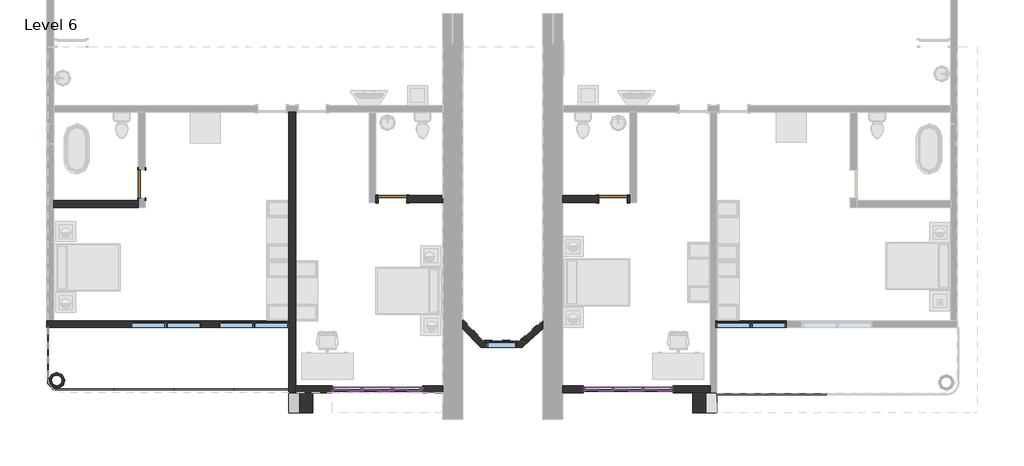
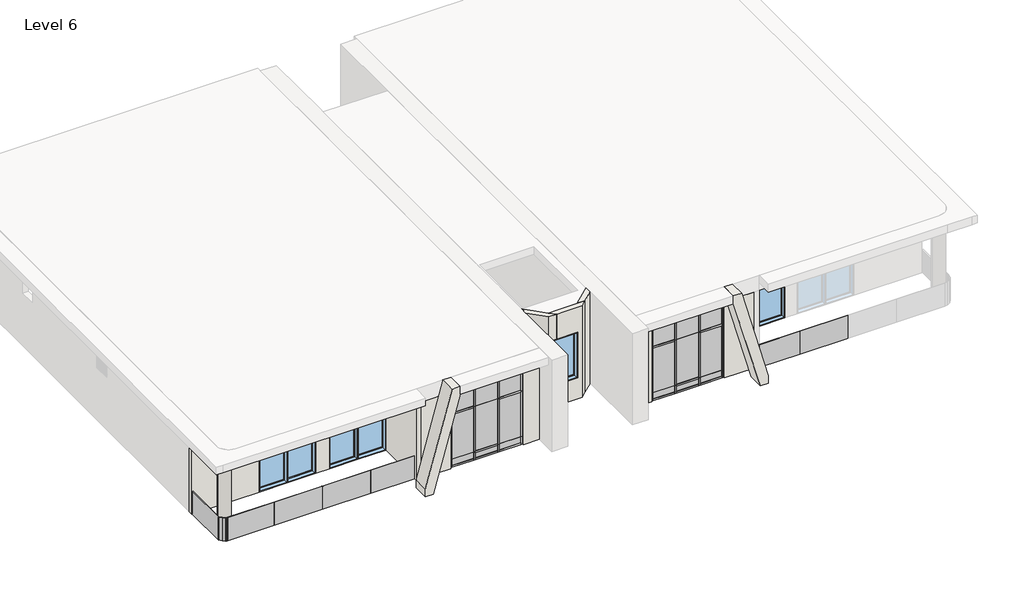
# One storey, part 1 of 3: 42 members, 29 plates, 16 walls, 7 windows, 3 doors.
"""IFC4 building model written with IfcOpenShell, lengths in millimetres."""

from ifc_helpers import new_model, si_unit, point, frame, frame_2d, origin, place, context, project, spatial, polyline, circle_curve, trimmed, segment, composite_curve, outline, extrude, faceted_brep, transform, mapped, element, save
from components import door_2703ae13, door_10fd3a06, member_c17f1be2, member_ad567e07, member_d2e7e466, member_7db1855a, member_75d1e245, member_d60e8053, member_3c3dc66a, member_2fae0574, member_410c6227, member_73c23c35, system_panel_glazed_38d54ecf, system_panel_glazed_fbb6c980, system_panel_glazed_4137532c, system_panel_glazed_6230de04, system_panel_glazed_a79f7f85, system_panel_glazed_9a5ea490, system_panel_glazed_95be5de7, system_panel_glazed_ffe51582, system_panel_glazed_8f95e3f6, system_panel_glazed_836907cd, system_panel_glazed_688a65a2, system_panel_glazed_c1a1c740, system_panel_glazed_22bcd51f, system_panel_glazed_4be86f7f, window_9a779fa2, window_1a213a25

model = new_model("IFC4")

# Units and contexts
model_context = context("Model", 3, world=origin())
ifc_project = project(units=[si_unit("LENGTHUNIT", "METRE", prefix="MILLI")], contexts=[model_context])

# Site, building, storey
site = spatial("IfcSite", under=ifc_project)
building = spatial("IfcBuilding", under=site)
storey = spatial("IfcBuildingStorey", under=building, Name="Level 6", Elevation=18288.0)

# Doors
placement = place(None, origin())
door_shape = door_2703ae13(model_context)
element("IfcDoor", 1, ObjectType="Door-Single-Panel.0001 : 34\" x 80\"", at=placement, inside=storey, context=model_context, shape_type="MappedRepresentation", body=[
    mapped(door_shape, transform((-15765.9987704, -441.9241442, 18288.0), x_axis=(0.0, -1.0, 0.0), y_axis=(1.0, 0.0, 0.0), z_axis=(0.0, 0.0, 1.0))),
])
element("IfcDoor", 2, ObjectType="Door-Single-Panel.0001 : 34\" x 80\"", at=placement, inside=storey, context=model_context, shape_type="MappedRepresentation", body=[
    mapped(door_shape, transform((-8145.9987704, -899.1241442, 18288.0), x_axis=(-1.0, 0.0, 0.0), y_axis=(0.0, -1.0, 0.0), z_axis=(0.0, 0.0, 1.0))),
])
door_2_shape = door_10fd3a06(model_context)
element("IfcDoor", 3, ObjectType="Door-Single-Panel.0001 : 34\" x 80\"", at=placement, inside=storey, context=model_context, shape_type="MappedRepresentation", body=[
    mapped(door_2_shape, transform((-1440.3987704, -899.1241442, 18288.0), x_axis=(1.0, 0.0, 0.0), y_axis=(0.0, 1.0, 0.0), z_axis=(0.0, 0.0, 1.0))),
])

# Members
member_shape = member_c17f1be2(model_context)
element("IfcMember", 4, ObjectType="Rectangular Mullion : 2.5\" x 5\" rectangular", at=placement, inside=storey, context=model_context, shape_type="MappedRepresentation", body=[
    mapped(member_shape, transform((-9911.2987704, -6690.3241442, 21336.0), x_axis=(0.0, 0.0, 1.0), y_axis=(0.0, 1.0, 0.0), z_axis=(-1.0, 0.0, 0.0))),
])
element("IfcMember", 5, ObjectType="Rectangular Mullion : 2.5\" x 5\" rectangular", at=placement, inside=storey, context=model_context, shape_type="MappedRepresentation", body=[
    mapped(member_shape, transform((-8114.2487704, -6690.3241442, 21336.0), x_axis=(0.0, 0.0, 1.0), y_axis=(0.0, 1.0, 0.0), z_axis=(-1.0, 0.0, 0.0))),
])
element("IfcMember", 6, ObjectType="Rectangular Mullion : 2.5\" x 5\" rectangular", at=placement, inside=storey, context=model_context, shape_type="MappedRepresentation", body=[
    mapped(member_shape, transform((-2291.2987704, -6690.3241442, 21336.0), x_axis=(0.0, 0.0, 1.0), y_axis=(0.0, 1.0, 0.0), z_axis=(-1.0, 0.0, 0.0))),
])
element("IfcMember", 7, ObjectType="Rectangular Mullion : 2.5\" x 5\" rectangular", at=placement, inside=storey, context=model_context, shape_type="MappedRepresentation", body=[
    mapped(member_shape, transform((-494.2487704, -6690.3241442, 21336.0), x_axis=(0.0, 0.0, 1.0), y_axis=(0.0, 1.0, 0.0), z_axis=(-1.0, 0.0, 0.0))),
])
element("IfcMember", 8, ObjectType="Rectangular Mullion : 2.5\" x 5\" rectangular", at=placement, inside=storey, context=model_context, shape_type="MappedRepresentation", body=[
    mapped(member_shape, transform((-7295.0987704, -6690.3241442, 18288.0), x_axis=(0.0, 0.0, -1.0), y_axis=(0.0, 1.0, 0.0), z_axis=(1.0, 0.0, 0.0))),
])
element("IfcMember", 9, ObjectType="Rectangular Mullion : 2.5\" x 5\" rectangular", at=placement, inside=storey, context=model_context, shape_type="MappedRepresentation", body=[
    mapped(member_shape, transform((-9092.1487704, -6690.3241442, 18288.0), x_axis=(0.0, 0.0, -1.0), y_axis=(0.0, 1.0, 0.0), z_axis=(1.0, 0.0, 0.0))),
])
element("IfcMember", 10, ObjectType="Rectangular Mullion : 2.5\" x 5\" rectangular", at=placement, inside=storey, context=model_context, shape_type="MappedRepresentation", body=[
    mapped(member_shape, transform((324.9012296, -6690.3241442, 18288.0), x_axis=(0.0, 0.0, -1.0), y_axis=(0.0, 1.0, 0.0), z_axis=(1.0, 0.0, 0.0))),
])
element("IfcMember", 11, ObjectType="Rectangular Mullion : 2.5\" x 5\" rectangular", at=placement, inside=storey, context=model_context, shape_type="MappedRepresentation", body=[
    mapped(member_shape, transform((-1472.1487704, -6690.3241442, 18288.0), x_axis=(0.0, 0.0, -1.0), y_axis=(0.0, 1.0, 0.0), z_axis=(1.0, 0.0, 0.0))),
])
member_2_shape = member_ad567e07(model_context)
element("IfcMember", 12, ObjectType="Rectangular Mullion : 2.5\" x 5\" rectangular", at=placement, inside=storey, context=model_context, shape_type="MappedRepresentation", body=[
    mapped(member_2_shape, transform((-8114.2487704, -6690.3241442, 20421.6), x_axis=(0.0, 0.0, 1.0), y_axis=(0.0, 1.0, 0.0), z_axis=(-1.0, 0.0, 0.0))),
])
element("IfcMember", 13, ObjectType="Rectangular Mullion : 2.5\" x 5\" rectangular", at=placement, inside=storey, context=model_context, shape_type="MappedRepresentation", body=[
    mapped(member_2_shape, transform((-9911.2987704, -6690.3241442, 20421.6), x_axis=(0.0, 0.0, 1.0), y_axis=(0.0, 1.0, 0.0), z_axis=(-1.0, 0.0, 0.0))),
])
element("IfcMember", 14, ObjectType="Rectangular Mullion : 2.5\" x 5\" rectangular", at=placement, inside=storey, context=model_context, shape_type="MappedRepresentation", body=[
    mapped(member_2_shape, transform((-494.2487704, -6690.3241442, 20421.6), x_axis=(0.0, 0.0, 1.0), y_axis=(0.0, 1.0, 0.0), z_axis=(-1.0, 0.0, 0.0))),
])
element("IfcMember", 15, ObjectType="Rectangular Mullion : 2.5\" x 5\" rectangular", at=placement, inside=storey, context=model_context, shape_type="MappedRepresentation", body=[
    mapped(member_2_shape, transform((-2291.2987704, -6690.3241442, 20421.6), x_axis=(0.0, 0.0, 1.0), y_axis=(0.0, 1.0, 0.0), z_axis=(-1.0, 0.0, 0.0))),
])
member_3_shape = member_d2e7e466(model_context)
element("IfcMember", 16, ObjectType="Rectangular Mullion : 2.5\" x 5\" rectangular", at=placement, inside=storey, context=model_context, shape_type="MappedRepresentation", body=[
    mapped(member_3_shape, transform((-8177.7487704, -6690.3241442, 18288.0), x_axis=(0.0, 0.0, -1.0), y_axis=(0.0, 1.0, 0.0), z_axis=(1.0, 0.0, 0.0))),
])
element("IfcMember", 17, ObjectType="Rectangular Mullion : 2.5\" x 5\" rectangular", at=placement, inside=storey, context=model_context, shape_type="MappedRepresentation", body=[
    mapped(member_3_shape, transform((-557.7487704, -6690.3241442, 18288.0), x_axis=(0.0, 0.0, -1.0), y_axis=(0.0, 1.0, 0.0), z_axis=(1.0, 0.0, 0.0))),
])
member_4_shape = member_7db1855a(model_context)
element("IfcMember", 18, ObjectType="Rectangular Mullion : 2.5\" x 5\" rectangular", at=placement, inside=storey, context=model_context, shape_type="MappedRepresentation", body=[
    mapped(member_4_shape, transform((-9028.6487704, -6690.3241442, 18592.8), x_axis=(0.0, 0.0, 1.0), y_axis=(0.0, 1.0, 0.0), z_axis=(-1.0, 0.0, 0.0))),
])
element("IfcMember", 19, ObjectType="Rectangular Mullion : 2.5\" x 5\" rectangular", at=placement, inside=storey, context=model_context, shape_type="MappedRepresentation", body=[
    mapped(member_4_shape, transform((-1408.6487704, -6690.3241442, 18592.8), x_axis=(0.0, 0.0, 1.0), y_axis=(0.0, 1.0, 0.0), z_axis=(-1.0, 0.0, 0.0))),
])
element("IfcMember", 20, ObjectType="Rectangular Mullion : 2.5\" x 5\" rectangular", at=placement, inside=storey, context=model_context, shape_type="MappedRepresentation", body=[
    mapped(member_3_shape, transform((-9028.6487704, -6690.3241442, 21336.0), x_axis=(0.0, 0.0, 1.0), y_axis=(0.0, 1.0, 0.0), z_axis=(-1.0, 0.0, 0.0))),
])
element("IfcMember", 21, ObjectType="Rectangular Mullion : 2.5\" x 5\" rectangular", at=placement, inside=storey, context=model_context, shape_type="MappedRepresentation", body=[
    mapped(member_3_shape, transform((-1408.6487704, -6690.3241442, 21336.0), x_axis=(0.0, 0.0, 1.0), y_axis=(0.0, 1.0, 0.0), z_axis=(-1.0, 0.0, 0.0))),
])
member_5_shape = member_75d1e245(model_context)
element("IfcMember", 22, ObjectType="Rectangular Mullion : 2.5\" x 5\" rectangular", at=placement, inside=storey, context=model_context, shape_type="MappedRepresentation", body=[
    mapped(member_5_shape, transform((-8145.9987704, -6690.3241442, 18288.0), x_axis=(-1.0, 0.0, 0.0), y_axis=(0.0, 1.0, 0.0), z_axis=(0.0, 0.0, -1.0))),
])
element("IfcMember", 23, ObjectType="Rectangular Mullion : 2.5\" x 5\" rectangular", at=placement, inside=storey, context=model_context, shape_type="MappedRepresentation", body=[
    mapped(member_5_shape, transform((-9060.3987704, -6690.3241442, 18288.0), x_axis=(-1.0, 0.0, 0.0), y_axis=(0.0, 1.0, 0.0), z_axis=(0.0, 0.0, -1.0))),
])
element("IfcMember", 24, ObjectType="Rectangular Mullion : 2.5\" x 5\" rectangular", at=placement, inside=storey, context=model_context, shape_type="MappedRepresentation", body=[
    mapped(member_5_shape, transform((-525.9987704, -6690.3241442, 18288.0), x_axis=(-1.0, 0.0, 0.0), y_axis=(0.0, 1.0, 0.0), z_axis=(0.0, 0.0, -1.0))),
])
element("IfcMember", 25, ObjectType="Rectangular Mullion : 2.5\" x 5\" rectangular", at=placement, inside=storey, context=model_context, shape_type="MappedRepresentation", body=[
    mapped(member_5_shape, transform((-1440.3987704, -6690.3241442, 18288.0), x_axis=(-1.0, 0.0, 0.0), y_axis=(0.0, 1.0, 0.0), z_axis=(0.0, 0.0, -1.0))),
])
member_6_shape = member_d60e8053(model_context)
element("IfcMember", 26, ObjectType="Rectangular Mullion : 2.5\" x 5\" rectangular", at=placement, inside=storey, context=model_context, shape_type="MappedRepresentation", body=[
    mapped(member_6_shape, transform((-8145.9987704, -6690.3241442, 18592.8), x_axis=(-1.0, 0.0, 0.0), y_axis=(0.0, 1.0, 0.0), z_axis=(0.0, 0.0, -1.0))),
])
element("IfcMember", 27, ObjectType="Rectangular Mullion : 2.5\" x 5\" rectangular", at=placement, inside=storey, context=model_context, shape_type="MappedRepresentation", body=[
    mapped(member_6_shape, transform((-9060.3987704, -6690.3241442, 18592.8), x_axis=(-1.0, 0.0, 0.0), y_axis=(0.0, 1.0, 0.0), z_axis=(0.0, 0.0, -1.0))),
])
element("IfcMember", 28, ObjectType="Rectangular Mullion : 2.5\" x 5\" rectangular", at=placement, inside=storey, context=model_context, shape_type="MappedRepresentation", body=[
    mapped(member_6_shape, transform((-525.9987704, -6690.3241442, 18592.8), x_axis=(-1.0, 0.0, 0.0), y_axis=(0.0, 1.0, 0.0), z_axis=(0.0, 0.0, -1.0))),
])
element("IfcMember", 29, ObjectType="Rectangular Mullion : 2.5\" x 5\" rectangular", at=placement, inside=storey, context=model_context, shape_type="MappedRepresentation", body=[
    mapped(member_6_shape, transform((-1440.3987704, -6690.3241442, 18592.8), x_axis=(-1.0, 0.0, 0.0), y_axis=(0.0, 1.0, 0.0), z_axis=(0.0, 0.0, -1.0))),
])
member_7_shape = member_3c3dc66a(model_context)
element("IfcMember", 30, ObjectType="Rectangular Mullion : 2.5\" x 5\" rectangular", at=placement, inside=storey, context=model_context, shape_type="MappedRepresentation", body=[
    mapped(member_7_shape, transform((-9974.7987704, -6690.3241442, 18288.0), x_axis=(-1.0, 0.0, 0.0), y_axis=(0.0, 1.0, 0.0), z_axis=(0.0, 0.0, -1.0))),
])
element("IfcMember", 31, ObjectType="Rectangular Mullion : 2.5\" x 5\" rectangular", at=placement, inside=storey, context=model_context, shape_type="MappedRepresentation", body=[
    mapped(member_7_shape, transform((-2354.7987704, -6690.3241442, 18288.0), x_axis=(-1.0, 0.0, 0.0), y_axis=(0.0, 1.0, 0.0), z_axis=(0.0, 0.0, -1.0))),
])
member_8_shape = member_2fae0574(model_context)
element("IfcMember", 32, ObjectType="Rectangular Mullion : 2.5\" x 5\" rectangular", at=placement, inside=storey, context=model_context, shape_type="MappedRepresentation", body=[
    mapped(member_8_shape, transform((-9974.7987704, -6690.3241442, 18592.8), x_axis=(-1.0, 0.0, 0.0), y_axis=(0.0, 1.0, 0.0), z_axis=(0.0, 0.0, -1.0))),
])
element("IfcMember", 33, ObjectType="Rectangular Mullion : 2.5\" x 5\" rectangular", at=placement, inside=storey, context=model_context, shape_type="MappedRepresentation", body=[
    mapped(member_8_shape, transform((-2354.7987704, -6690.3241442, 18592.8), x_axis=(-1.0, 0.0, 0.0), y_axis=(0.0, 1.0, 0.0), z_axis=(0.0, 0.0, -1.0))),
])
element("IfcMember", 34, ObjectType="Rectangular Mullion : 2.5\" x 5\" rectangular", at=placement, inside=storey, context=model_context, shape_type="MappedRepresentation", body=[
    mapped(member_8_shape, transform((-7231.5987704, -6690.3241442, 20421.6), x_axis=(1.0, 0.0, 0.0), y_axis=(0.0, 1.0, 0.0), z_axis=(0.0, 0.0, 1.0))),
])
element("IfcMember", 35, ObjectType="Rectangular Mullion : 2.5\" x 5\" rectangular", at=placement, inside=storey, context=model_context, shape_type="MappedRepresentation", body=[
    mapped(member_8_shape, transform((388.4012296, -6690.3241442, 20421.6), x_axis=(1.0, 0.0, 0.0), y_axis=(0.0, 1.0, 0.0), z_axis=(0.0, 0.0, 1.0))),
])
element("IfcMember", 36, ObjectType="Rectangular Mullion : 2.5\" x 5\" rectangular", at=placement, inside=storey, context=model_context, shape_type="MappedRepresentation", body=[
    mapped(member_7_shape, transform((-7231.5987704, -6690.3241442, 18592.8), x_axis=(1.0, 0.0, 0.0), y_axis=(0.0, 1.0, 0.0), z_axis=(0.0, 0.0, 1.0))),
])
element("IfcMember", 37, ObjectType="Rectangular Mullion : 2.5\" x 5\" rectangular", at=placement, inside=storey, context=model_context, shape_type="MappedRepresentation", body=[
    mapped(member_7_shape, transform((388.4012296, -6690.3241442, 18592.8), x_axis=(1.0, 0.0, 0.0), y_axis=(0.0, 1.0, 0.0), z_axis=(0.0, 0.0, 1.0))),
])
member_9_shape = member_410c6227(model_context)
element("IfcMember", 38, ObjectType="Rectangular Mullion : 2.5\" x 5\" rectangular", at=placement, inside=storey, context=model_context, shape_type="MappedRepresentation", body=[
    mapped(member_9_shape, transform((-8145.9987704, -6690.3241442, 20421.6), x_axis=(-1.0, 0.0, 0.0), y_axis=(0.0, 1.0, 0.0), z_axis=(0.0, 0.0, -1.0))),
])
element("IfcMember", 39, ObjectType="Rectangular Mullion : 2.5\" x 5\" rectangular", at=placement, inside=storey, context=model_context, shape_type="MappedRepresentation", body=[
    mapped(member_9_shape, transform((-9060.3987704, -6690.3241442, 20421.6), x_axis=(-1.0, 0.0, 0.0), y_axis=(0.0, 1.0, 0.0), z_axis=(0.0, 0.0, -1.0))),
])
element("IfcMember", 40, ObjectType="Rectangular Mullion : 2.5\" x 5\" rectangular", at=placement, inside=storey, context=model_context, shape_type="MappedRepresentation", body=[
    mapped(member_9_shape, transform((-525.9987704, -6690.3241442, 20421.6), x_axis=(-1.0, 0.0, 0.0), y_axis=(0.0, 1.0, 0.0), z_axis=(0.0, 0.0, -1.0))),
])
element("IfcMember", 41, ObjectType="Rectangular Mullion : 2.5\" x 5\" rectangular", at=placement, inside=storey, context=model_context, shape_type="MappedRepresentation", body=[
    mapped(member_9_shape, transform((-1440.3987704, -6690.3241442, 20421.6), x_axis=(-1.0, 0.0, 0.0), y_axis=(0.0, 1.0, 0.0), z_axis=(0.0, 0.0, -1.0))),
])
member_10_shape = member_73c23c35(model_context)
element("IfcMember", 42, ObjectType="Rectangular Mullion : 2.5\" x 5\" rectangular", at=placement, inside=storey, context=model_context, shape_type="MappedRepresentation", body=[
    mapped(member_10_shape, transform((-7231.5987704, -6690.3241442, 21336.0), x_axis=(1.0, 0.0, 0.0), y_axis=(0.0, 1.0, 0.0), z_axis=(0.0, 0.0, 1.0))),
])
element("IfcMember", 43, ObjectType="Rectangular Mullion : 2.5\" x 5\" rectangular", at=placement, inside=storey, context=model_context, shape_type="MappedRepresentation", body=[
    mapped(member_10_shape, transform((388.4012296, -6690.3241442, 21336.0), x_axis=(1.0, 0.0, 0.0), y_axis=(0.0, 1.0, 0.0), z_axis=(0.0, 0.0, 1.0))),
])
element("IfcMember", 44, ObjectType="Rectangular Mullion : 2.5\" x 5\" rectangular", at=placement, inside=storey, context=model_context, shape_type="MappedRepresentation", body=[
    mapped(member_10_shape, transform((-9974.7987704, -6690.3241442, 20421.6), x_axis=(-1.0, 0.0, 0.0), y_axis=(0.0, 1.0, 0.0), z_axis=(0.0, 0.0, -1.0))),
])
element("IfcMember", 45, ObjectType="Rectangular Mullion : 2.5\" x 5\" rectangular", at=placement, inside=storey, context=model_context, shape_type="MappedRepresentation", body=[
    mapped(member_10_shape, transform((-2354.7987704, -6690.3241442, 20421.6), x_axis=(-1.0, 0.0, 0.0), y_axis=(0.0, 1.0, 0.0), z_axis=(0.0, 0.0, -1.0))),
])

# Plates
system_panel_glazed_shape = system_panel_glazed_38d54ecf(model_context)
element("IfcPlate", 46, ObjectType="System Panel : Glazed", at=placement, inside=storey, context=model_context, shape_type="MappedRepresentation", body=[
    mapped(system_panel_glazed_shape, transform((-8603.1987704, -6690.3241442, 18624.55), x_axis=(-1.0, 0.0, 0.0), y_axis=(0.0, -1.0, 0.0), z_axis=(0.0, 0.0, 1.0))),
])
element("IfcPlate", 47, ObjectType="System Panel : Glazed", at=placement, inside=storey, context=model_context, shape_type="MappedRepresentation", body=[
    mapped(system_panel_glazed_shape, transform((-983.1987704, -6690.3241442, 18624.55), x_axis=(-1.0, 0.0, 0.0), y_axis=(0.0, -1.0, 0.0), z_axis=(0.0, 0.0, 1.0))),
])
system_panel_glazed_2_shape = system_panel_glazed_fbb6c980(model_context)
element("IfcPlate", 48, ObjectType="System Panel : Glazed", at=placement, inside=storey, context=model_context, shape_type="MappedRepresentation", body=[
    mapped(system_panel_glazed_2_shape, transform((-8603.1987704, -6690.3241442, 18351.5), x_axis=(-1.0, 0.0, 0.0), y_axis=(0.0, -1.0, 0.0), z_axis=(0.0, 0.0, 1.0))),
])
element("IfcPlate", 49, ObjectType="System Panel : Glazed", at=placement, inside=storey, context=model_context, shape_type="MappedRepresentation", body=[
    mapped(system_panel_glazed_2_shape, transform((-983.1987704, -6690.3241442, 18351.5), x_axis=(-1.0, 0.0, 0.0), y_axis=(0.0, -1.0, 0.0), z_axis=(0.0, 0.0, 1.0))),
])
system_panel_glazed_3_shape = system_panel_glazed_4137532c(model_context)
element("IfcPlate", 50, ObjectType="System Panel : Glazed", at=placement, inside=storey, context=model_context, shape_type="MappedRepresentation", body=[
    mapped(system_panel_glazed_3_shape, transform((-7704.6737704, -6690.3241442, 18351.5), x_axis=(-1.0, 0.0, 0.0), y_axis=(0.0, -1.0, 0.0), z_axis=(0.0, 0.0, 1.0))),
])
element("IfcPlate", 51, ObjectType="System Panel : Glazed", at=placement, inside=storey, context=model_context, shape_type="MappedRepresentation", body=[
    mapped(system_panel_glazed_3_shape, transform((-9501.7237704, -6690.3241442, 18351.5), x_axis=(-1.0, 0.0, 0.0), y_axis=(0.0, -1.0, 0.0), z_axis=(0.0, 0.0, 1.0))),
])
element("IfcPlate", 52, ObjectType="System Panel : Glazed", at=placement, inside=storey, context=model_context, shape_type="MappedRepresentation", body=[
    mapped(system_panel_glazed_3_shape, transform((-84.6737704, -6690.3241442, 18351.5), x_axis=(-1.0, 0.0, 0.0), y_axis=(0.0, -1.0, 0.0), z_axis=(0.0, 0.0, 1.0))),
])
element("IfcPlate", 53, ObjectType="System Panel : Glazed", at=placement, inside=storey, context=model_context, shape_type="MappedRepresentation", body=[
    mapped(system_panel_glazed_3_shape, transform((-1881.7237704, -6690.3241442, 18351.5), x_axis=(-1.0, 0.0, 0.0), y_axis=(0.0, -1.0, 0.0), z_axis=(0.0, 0.0, 1.0))),
])
system_panel_glazed_4_shape = system_panel_glazed_6230de04(model_context)
element("IfcPlate", 54, ObjectType="System Panel : Glazed", at=placement, inside=storey, context=model_context, shape_type="MappedRepresentation", body=[
    mapped(system_panel_glazed_4_shape, transform((-7704.6737704, -6690.3241442, 18592.8), x_axis=(-1.0, 0.0, 0.0), y_axis=(0.0, -1.0, 0.0), z_axis=(0.0, 0.0, 1.0))),
])
element("IfcPlate", 55, ObjectType="System Panel : Glazed", at=placement, inside=storey, context=model_context, shape_type="MappedRepresentation", body=[
    mapped(system_panel_glazed_4_shape, transform((-9501.7237704, -6690.3241442, 18592.8), x_axis=(-1.0, 0.0, 0.0), y_axis=(0.0, -1.0, 0.0), z_axis=(0.0, 0.0, 1.0))),
])
element("IfcPlate", 56, ObjectType="System Panel : Glazed", at=placement, inside=storey, context=model_context, shape_type="MappedRepresentation", body=[
    mapped(system_panel_glazed_4_shape, transform((-84.6737704, -6690.3241442, 18592.8), x_axis=(-1.0, 0.0, 0.0), y_axis=(0.0, -1.0, 0.0), z_axis=(0.0, 0.0, 1.0))),
])
element("IfcPlate", 57, ObjectType="System Panel : Glazed", at=placement, inside=storey, context=model_context, shape_type="MappedRepresentation", body=[
    mapped(system_panel_glazed_4_shape, transform((-1881.7237704, -6690.3241442, 18592.8), x_axis=(-1.0, 0.0, 0.0), y_axis=(0.0, -1.0, 0.0), z_axis=(0.0, 0.0, 1.0))),
])
system_panel_glazed_5_shape = system_panel_glazed_a79f7f85(model_context)
element("IfcPlate", 58, ObjectType="System Panel : Glazed", at=placement, inside=storey, context=model_context, shape_type="MappedRepresentation", body=[
    mapped(system_panel_glazed_5_shape, transform((-7704.6737704, -6690.3241442, 20453.35), x_axis=(-1.0, 0.0, 0.0), y_axis=(0.0, -1.0, 0.0), z_axis=(0.0, 0.0, 1.0))),
])
element("IfcPlate", 59, ObjectType="System Panel : Glazed", at=placement, inside=storey, context=model_context, shape_type="MappedRepresentation", body=[
    mapped(system_panel_glazed_5_shape, transform((-9501.7237704, -6690.3241442, 20453.35), x_axis=(-1.0, 0.0, 0.0), y_axis=(0.0, -1.0, 0.0), z_axis=(0.0, 0.0, 1.0))),
])
element("IfcPlate", 60, ObjectType="System Panel : Glazed", at=placement, inside=storey, context=model_context, shape_type="MappedRepresentation", body=[
    mapped(system_panel_glazed_5_shape, transform((-84.6737704, -6690.3241442, 20453.35), x_axis=(-1.0, 0.0, 0.0), y_axis=(0.0, -1.0, 0.0), z_axis=(0.0, 0.0, 1.0))),
])
element("IfcPlate", 61, ObjectType="System Panel : Glazed", at=placement, inside=storey, context=model_context, shape_type="MappedRepresentation", body=[
    mapped(system_panel_glazed_5_shape, transform((-1881.7237704, -6690.3241442, 20453.35), x_axis=(-1.0, 0.0, 0.0), y_axis=(0.0, -1.0, 0.0), z_axis=(0.0, 0.0, 1.0))),
])
system_panel_glazed_6_shape = system_panel_glazed_9a5ea490(model_context)
element("IfcPlate", 62, ObjectType="System Panel : Glazed", at=placement, inside=storey, context=model_context, shape_type="MappedRepresentation", body=[
    mapped(system_panel_glazed_6_shape, transform((-8603.1987704, -6690.3241442, 20421.6), x_axis=(-1.0, 0.0, 0.0), y_axis=(0.0, -1.0, 0.0), z_axis=(0.0, 0.0, 1.0))),
])
element("IfcPlate", 63, ObjectType="System Panel : Glazed", at=placement, inside=storey, context=model_context, shape_type="MappedRepresentation", body=[
    mapped(system_panel_glazed_6_shape, transform((-983.1987704, -6690.3241442, 20421.6), x_axis=(-1.0, 0.0, 0.0), y_axis=(0.0, -1.0, 0.0), z_axis=(0.0, 0.0, 1.0))),
])
system_panel_glazed_7_shape = system_panel_glazed_95be5de7(model_context)
element("IfcPlate", 64, ObjectType="System Panel : Glazed", at=placement, inside=storey, context=model_context, shape_type="MappedRepresentation", body=[
    mapped(system_panel_glazed_7_shape, transform((-15707.2305745, -6723.6923401, 18288.0), x_axis=(1.0, 0.0, 0.0), y_axis=(0.0, 1.0, 0.0), z_axis=(0.0, 0.0, 1.0))),
])
element("IfcPlate", 65, ObjectType="System Panel : Glazed", at=placement, inside=storey, context=model_context, shape_type="MappedRepresentation", body=[
    mapped(system_panel_glazed_7_shape, transform((-13878.4305745, -6723.6923401, 18288.0), x_axis=(1.0, 0.0, 0.0), y_axis=(0.0, 1.0, 0.0), z_axis=(0.0, 0.0, 1.0))),
])
element("IfcPlate", 66, ObjectType="System Panel : Glazed", at=placement, inside=storey, context=model_context, shape_type="MappedRepresentation", body=[
    mapped(system_panel_glazed_7_shape, transform((4129.1120092, -6810.4133646, 18288.0), x_axis=(-1.0, 0.0, 0.0), y_axis=(0.0, -1.0, 0.0), z_axis=(0.0, 0.0, 1.0))),
])
system_panel_glazed_8_shape = system_panel_glazed_ffe51582(model_context)
element("IfcPlate", 67, ObjectType="System Panel : Glazed", at=placement, inside=storey, context=model_context, shape_type="MappedRepresentation", body=[
    mapped(system_panel_glazed_8_shape, transform((-18451.9713429, -6722.1515718, 18288.0), x_axis=(0.7071067811865462, -0.7071067811865488, 0.0), y_axis=(0.7071067811865488, 0.7071067811865462, 0.0), z_axis=(0.0, 0.0, 1.0))),
])
system_panel_glazed_9_shape = system_panel_glazed_8f95e3f6(model_context)
element("IfcPlate", 68, ObjectType="System Panel : Glazed", at=placement, inside=storey, context=model_context, shape_type="MappedRepresentation", body=[
    mapped(system_panel_glazed_9_shape, transform((-18648.8987704, -5667.9741442, 18288.0), x_axis=(0.0, -1.0, 0.0), y_axis=(1.0, 0.0, 0.0), z_axis=(0.0, 0.0, 1.0))),
])
system_panel_glazed_10_shape = system_panel_glazed_836907cd(model_context)
element("IfcPlate", 69, ObjectType="System Panel : Glazed", at=placement, inside=storey, context=model_context, shape_type="MappedRepresentation", body=[
    mapped(system_panel_glazed_10_shape, transform((-18418.6805745, -6723.6923401, 18288.0), x_axis=(1.0, 0.0, 0.0), y_axis=(0.0, 1.0, 0.0), z_axis=(0.0, 0.0, 1.0))),
])
system_panel_glazed_11_shape = system_panel_glazed_688a65a2(model_context)
element("IfcPlate", 70, ObjectType="System Panel : Glazed", at=placement, inside=storey, context=model_context, shape_type="MappedRepresentation", body=[
    mapped(system_panel_glazed_11_shape, transform((-12129.8146725, -6723.6923401, 18288.0), x_axis=(1.0, 0.0, 0.0), y_axis=(0.0, 1.0, 0.0), z_axis=(0.0, 0.0, 1.0))),
])
system_panel_glazed_12_shape = system_panel_glazed_c1a1c740(model_context)
element("IfcPlate", 71, ObjectType="System Panel : Glazed", at=placement, inside=storey, context=model_context, shape_type="MappedRepresentation", body=[
    mapped(system_panel_glazed_12_shape, transform((-17504.2805745, -6723.6923401, 18288.0), x_axis=(1.0, 0.0, 0.0), y_axis=(0.0, 1.0, 0.0), z_axis=(0.0, 0.0, 1.0))),
])
system_panel_glazed_13_shape = system_panel_glazed_22bcd51f(model_context)
element("IfcPlate", 72, ObjectType="System Panel : Glazed", at=placement, inside=storey, context=model_context, shape_type="MappedRepresentation", body=[
    mapped(system_panel_glazed_13_shape, transform((-18600.0521056, -6574.070809, 18288.0), x_axis=(0.7071067811865462, -0.7071067811865488, 0.0), y_axis=(0.7071067811865488, 0.7071067811865462, 0.0), z_axis=(0.0, 0.0, 1.0))),
])
element("IfcPlate", 73, ObjectType="System Panel : Glazed", at=placement, inside=storey, context=model_context, shape_type="MappedRepresentation", body=[
    mapped(system_panel_glazed_13_shape, transform((-18502.3587761, -6671.7641386, 18288.0), x_axis=(0.7071067811865462, -0.7071067811865488, 0.0), y_axis=(0.7071067811865488, 0.7071067811865462, 0.0), z_axis=(0.0, 0.0, 1.0))),
])
system_panel_glazed_14_shape = system_panel_glazed_4be86f7f(model_context)
element("IfcPlate", 74, ObjectType="System Panel : Glazed", at=placement, inside=storey, context=model_context, shape_type="MappedRepresentation", body=[
    mapped(system_panel_glazed_14_shape, transform((2460.5794118, -6810.4133646, 18288.0), x_axis=(-1.0, 0.0, 0.0), y_axis=(0.0, -1.0, 0.0), z_axis=(0.0, 0.0, 1.0))),
])

# Walls
element("IfcWall", 75, ObjectType="Generic - 3\" green 2", at=placement, inside=storey, context=model_context, shape_type="SweptSolid", body=[
    extrude(outline(composite_curve([segment(polyline([(-18518.7237704, -6418.8616442), (-18594.9237704, -6418.8616442)]), True, "CONTINUOUS"), segment(trimmed(circle_curve(frame_2d((-18353.6237704, -6418.8616442)), 241.3), [point((-18594.9237704, -6418.8616442))], [point((-18112.3237704, -6418.8616442))], False, "CARTESIAN"), True, "CONTINUOUS"), segment(polyline([(-18112.3237704, -6418.8616442), (-18188.5237704, -6418.8616442)]), True, "CONTINUOUS"), segment(trimmed(circle_curve(frame_2d((-18353.6237704, -6418.8616442)), 165.1), [point((-18188.5237704, -6418.8616442))], [point((-18518.7237704, -6418.8616442))], True, "CARTESIAN"), True, "CONTINUOUS")], self_intersect=False)), frame((0.0, 0.0, 18288.0), z_axis=(0.0, 0.0, 1.0), x_axis=(1.0, 0.0, 0.0)), (0.0, 0.0, 1.0), 3048.0),
])
element("IfcWall", 76, ObjectType="Generic - 3\" green 2", at=placement, inside=storey, context=model_context, shape_type="SweptSolid", body=[
    extrude(outline(composite_curve([segment(polyline([(-18188.5237704, -6418.8616442), (-18112.3237704, -6418.8616442)]), True, "CONTINUOUS"), segment(trimmed(circle_curve(frame_2d((-18353.6237704, -6418.8616442)), 241.3), [point((-18112.3237704, -6418.8616442))], [point((-18594.9237704, -6418.8616442))], False, "CARTESIAN"), True, "CONTINUOUS"), segment(polyline([(-18594.9237704, -6418.8616442), (-18518.7237704, -6418.8616442)]), True, "CONTINUOUS"), segment(trimmed(circle_curve(frame_2d((-18353.6237704, -6418.8616442)), 165.1), [point((-18518.7237704, -6418.8616442))], [point((-18188.5237704, -6418.8616442))], True, "CARTESIAN"), True, "CONTINUOUS")], self_intersect=False)), frame((0.0, 0.0, 18288.0), z_axis=(0.0, 0.0, 1.0), x_axis=(1.0, 0.0, 0.0)), (0.0, 0.0, 1.0), 3048.0),
])
element("IfcWall", 77, ObjectType="Generic - 8\" cream", at=placement, inside=storey, context=model_context, shape_type="Brep", body=[
    faceted_brep([(-11295.5987704, 1742.4758558, 18288.0), (-11295.5987704, -6791.9241442, 18288.0), (-11295.5987704, -6791.9241442, 21336.0), (-11295.5987704, -4810.7241442, 21336.0), (-11295.5987704, -4607.5241442, 21336.0), (-11295.5987704, 1742.4758558, 21336.0), (-11092.3987704, 1742.4758558, 18288.0), (-11092.3987704, 1742.4758558, 21336.0), (-11092.3987704, -6588.7241442, 21336.0), (-11092.3987704, -6791.9241442, 21336.0), (-11092.3987704, -6791.9241442, 18288.0), (-11092.3987704, -6588.7241442, 18288.0)], [[[0, 1, 2, 3, 4, 5]], [[6, 7, 8, 9, 10, 11]], [[1, 0, 6, 11, 10]], [[5, 4, 3, 2, 9, 8, 7]], [[0, 5, 7, 6]], [[2, 1, 10, 9]]]),
])
element("IfcWall", 78, ObjectType="Generic - 8\" cream", at=placement, inside=storey, context=model_context, shape_type="SweptSolid", body=[
    extrude(outline(polyline([(-18445.6987704, -949.9241442), (-15867.5987704, -949.9241442), (-15867.5987704, -1153.1241442), (-18445.6987704, -1153.1241442), (-18445.6987704, -949.9241442)])), frame((0.0, 0.0, 18288.0), z_axis=(0.0, 0.0, 1.0), x_axis=(1.0, 0.0, 0.0)), (0.0, 0.0, 1.0), 3048.0),
])
element("IfcWall", 79, ObjectType="Generic - 8\" cream", at=placement, inside=storey, context=model_context, shape_type="SweptSolid", body=[
    extrude(outline(polyline([(21336.0, -6621.9987704), (21336.0, -8653.9987704), (18288.0, -8653.9987704), (18288.0, -8577.7987704), (20320.0, -8577.7987704), (20320.0, -7714.1987704), (18288.0, -7714.1987704), (18288.0, -6621.9987704), (21336.0, -6621.9987704)])), frame((0.0, -1000.7241442, 0.0), z_axis=(0.0, 1.0, 0.0), x_axis=(0.0, 0.0, 1.0)), (0.0, 0.0, 1.0), 203.2),
])
element("IfcWall", 80, ObjectType="Generic - 8\" cream", at=placement, inside=storey, context=model_context, shape_type="Brep", body=[
    faceted_brep([(-18648.8987704, -4607.5241442, 21336.0), (-18445.6987704, -4607.5241442, 21336.0), (-11295.5987704, -4607.5241442, 21336.0), (-11295.5987704, -4607.5241442, 21031.2), (-13429.1987704, -4607.5241442, 21031.2), (-13429.1987704, -4607.5241442, 18288.0), (-13962.5987704, -4607.5241442, 18288.0), (-13962.5987704, -4607.5241442, 21031.2), (-16096.1987704, -4607.5241442, 21031.2), (-16096.1987704, -4607.5241442, 18288.0), (-18445.6987704, -4607.5241442, 18288.0), (-18648.8987704, -4607.5241442, 18288.0), (-11295.5987704, -4810.7241442, 21336.0), (-18648.8987704, -4810.7241442, 21336.0), (-18648.8987704, -4810.7241442, 18288.0), (-16096.1987704, -4810.7241442, 18288.0), (-16096.1987704, -4810.7241442, 21031.2), (-13962.5987704, -4810.7241442, 21031.2), (-13962.5987704, -4810.7241442, 18288.0), (-13429.1987704, -4810.7241442, 18288.0), (-13429.1987704, -4810.7241442, 21031.2), (-11295.5987704, -4810.7241442, 21031.2)], [[[0, 1, 2, 3, 4, 5, 6, 7, 8, 9, 10, 11]], [[12, 13, 14, 15, 16, 17, 18, 19, 20, 21]], [[14, 11, 10, 9, 15]], [[5, 19, 18, 6]], [[2, 1, 0, 13, 12]], [[2, 12, 21, 3]], [[0, 11, 14, 13]], [[3, 21, 20, 4]], [[4, 20, 19, 5]], [[17, 7, 6, 18]], [[7, 17, 16, 8]], [[8, 16, 15, 9]]]),
])
element("IfcWall", 81, ObjectType="Generic - 8\" cream", at=placement, inside=storey, context=model_context, shape_type="SweptSolid", body=[
    extrude(outline(polyline([(21336.0, -932.3987704), (21336.0, -2964.3987704), (18288.0, -2964.3987704), (18288.0, -1872.1987704), (20320.0, -1872.1987704), (20320.0, -1008.5987704), (18288.0, -1008.5987704), (18288.0, -932.3987704), (21336.0, -932.3987704)])), frame((0.0, -1000.7241442, 0.0), z_axis=(0.0, 1.0, 0.0), x_axis=(0.0, 0.0, 1.0)), (0.0, 0.0, 1.0), 203.2),
])
element("IfcWall", 82, ObjectType="Generic - 8\" cream", at=placement, inside=storey, context=model_context, shape_type="SweptSolid", body=[
    extrude(outline(polyline([(388.4012296, -6588.7241442), (1506.0012296, -6588.7241442), (1506.0012296, -6791.9241442), (388.4012296, -6791.9241442), (388.4012296, -6588.7241442)])), frame((0.0, 0.0, 18288.0), z_axis=(0.0, 0.0, 1.0), x_axis=(1.0, 0.0, 0.0)), (0.0, 0.0, 1.0), 3048.0),
])
element("IfcWall", 83, ObjectType="Generic - 8\" cream", at=placement, inside=storey, context=model_context, shape_type="SweptSolid", body=[
    extrude(outline(polyline([(-2354.7987704, -6791.9241442), (-2964.3987704, -6791.9241442), (-2964.3987704, -6588.7241442), (-2354.7987704, -6588.7241442), (-2354.7987704, -6791.9241442)])), frame((0.0, 0.0, 18288.0), z_axis=(0.0, 0.0, 1.0), x_axis=(1.0, 0.0, 0.0)), (0.0, 0.0, 1.0), 3048.0),
])
element("IfcWall", 84, ObjectType="Generic - 8\" cream", at=placement, inside=storey, context=model_context, shape_type="SweptSolid", body=[
    extrude(outline(polyline([(-9974.7987704, -6791.9241442), (-11092.3987704, -6791.9241442), (-11092.3987704, -6588.7241442), (-9974.7987704, -6588.7241442), (-9974.7987704, -6791.9241442)])), frame((0.0, 0.0, 18288.0), z_axis=(0.0, 0.0, 1.0), x_axis=(1.0, 0.0, 0.0)), (0.0, 0.0, 1.0), 3048.0),
])
element("IfcWall", 85, ObjectType="Generic - 8\" cream", at=placement, inside=storey, context=model_context, shape_type="SweptSolid", body=[
    extrude(outline(polyline([(-7231.5987704, -6588.7241442), (-6621.9987704, -6588.7241442), (-6621.9987704, -6791.9241442), (-7231.5987704, -6791.9241442), (-7231.5987704, -6588.7241442)])), frame((0.0, 0.0, 18288.0), z_axis=(0.0, 0.0, 1.0), x_axis=(1.0, 0.0, 0.0)), (0.0, 0.0, 1.0), 3048.0),
])
element("IfcWall", 86, ObjectType="Generic - 8\" green", at=placement, inside=storey, context=model_context, shape_type="Brep", body=[
    faceted_brep([(-6012.3987704, -4852.8082422, 18288.0), (-5458.7044276, -5406.502585, 18288.0), (-5458.7044276, -5406.502585, 21945.6), (-6012.3987704, -4852.8082422, 21945.6), (-5171.3362318, -5406.502585, 18288.0), (-5374.5362318, -5203.302585, 18288.0), (-6012.3987704, -4565.4400463, 18288.0), (-6012.3987704, -4565.4400463, 21945.6), (-5374.5362318, -5203.302585, 21945.6), (-5171.3362318, -5406.502585, 21945.6), (-5171.3362318, -5406.502585, 20955.0), (-5289.4901401, -5288.3486766, 20955.0), (-5289.4901401, -5288.3486766, 19126.2), (-5171.3362318, -5406.502585, 19126.2), (-5289.4901401, -5406.502585, 19126.2), (-5289.4901401, -5406.502585, 20955.0)], [[[0, 1, 2, 3]], [[4, 5, 6, 7, 8, 9, 10, 11, 12, 13]], [[1, 0, 6, 5, 4]], [[3, 2, 9, 8, 7]], [[0, 3, 7, 6]], [[2, 1, 4, 13, 14, 15, 10, 9]], [[12, 14, 13]], [[14, 12, 11, 15]], [[15, 11, 10]]]),
])
element("IfcWall", 87, ObjectType="Generic - 8\" green", at=placement, inside=storey, context=model_context, shape_type="Brep", body=[
    faceted_brep([(-5171.3362318, -5406.502585, 18288.0), (-4203.3343712, -5406.502585, 18288.0), (-4203.3343712, -5406.502585, 21945.6), (-5171.3362318, -5406.502585, 21945.6), (-5171.3362318, -5406.502585, 20955.0), (-4375.0901401, -5406.502585, 20955.0), (-4375.0901401, -5406.502585, 19126.2), (-5171.3362318, -5406.502585, 19126.2), (-3975.4820774, -5203.302585, 18288.0), (-4280.7801413, -5203.302585, 18288.0), (-5374.5362318, -5203.302585, 18288.0), (-5374.5362318, -5203.302585, 21945.6), (-4280.7801413, -5203.302585, 21945.6), (-3975.4820774, -5203.302585, 21945.6), (-4375.0901401, -5203.302585, 19126.2), (-4375.0901401, -5203.302585, 20955.0), (-5289.4901401, -5203.302585, 20955.0), (-5289.4901401, -5203.302585, 19126.2), (-5289.4901401, -5288.3486766, 19126.2), (-5289.4901401, -5288.3486766, 20955.0)], [[[0, 1, 2, 3, 4, 5, 6, 7]], [[8, 9, 10, 11, 12, 13], [14, 15, 16, 17]], [[1, 0, 10, 9, 8]], [[3, 2, 13, 12, 11]], [[3, 11, 10, 0, 7, 18, 19, 4]], [[2, 1, 8, 13]], [[5, 15, 14, 6]], [[6, 14, 17, 18, 7]], [[18, 17, 16, 19]], [[15, 5, 4, 19, 16]]]),
])
element("IfcWall", 88, ObjectType="Generic - 8\" green", at=placement, inside=storey, context=model_context, shape_type="SweptSolid", body=[
    extrude(outline(polyline([(-3573.9987704, -4845.2574382), (-3975.4820774, -5203.302585), (-4280.7801413, -5203.302585), (-3573.9987704, -4572.9908503), (-3573.9987704, -4845.2574382)])), frame((0.0, 0.0, 18288.0), z_axis=(0.0, 0.0, 1.0), x_axis=(1.0, 0.0, 0.0)), (0.0, 0.0, 1.0), 3657.6),
])
element("IfcWall", 89, ObjectType="Generic -2' white 2", at=placement, inside=storey, context=model_context, shape_type="SweptSolid", body=[
    extrude(outline(polyline([(21640.8, -9974.7987704), (21945.6, -9974.7987704), (21945.6, -10279.5987704), (18288.0, -11295.5987704), (17983.2, -11295.5987704), (17983.2, -10990.7987704), (21640.8, -9974.7987704)])), frame((0.0, -7401.5241442, 0.0), z_axis=(0.0, 1.0, 0.0), x_axis=(0.0, 0.0, 1.0)), (0.0, 0.0, 1.0), 609.6),
])
element("IfcWall", 90, ObjectType="Generic -2' white 2", at=placement, inside=storey, context=model_context, shape_type="SweptSolid", body=[
    extrude(outline(polyline([(21640.8, 385.6468143), (17983.2, 1401.6468143), (17983.2, 1706.4468143), (18288.0, 1706.4468143), (21945.6, 690.4468143), (21945.6, 385.6468143), (21640.8, 385.6468143)])), frame((0.0, -7401.5241442, 0.0), z_axis=(0.0, 1.0, 0.0), x_axis=(0.0, 0.0, 1.0)), (0.0, 0.0, 1.0), 609.6),
])

# Windows
window_shape = window_9a779fa2(model_context)
element("IfcWindow", 91, ObjectType="Fixed : 36\" x 72\"", at=placement, inside=storey, context=model_context, shape_type="MappedRepresentation", body=[
    mapped(window_shape, transform((-4794.1901401, -5304.902585, 18821.4), x_axis=(1.0, 0.0, 0.0), y_axis=(0.0, 1.0, 0.0), z_axis=(0.0, 0.0, 1.0))),
])
window_2_shape = window_1a213a25(model_context)
element("IfcWindow", 92, ObjectType="Fixed : 36\" x 72\" 2", at=placement, inside=storey, context=model_context, shape_type="MappedRepresentation", body=[
    mapped(window_2_shape, transform((-11790.8987704, -4709.1241442, 17983.2), x_axis=(1.0, 0.0, 0.0), y_axis=(0.0, 1.0, 0.0), z_axis=(0.0, 0.0, 1.0))),
])
element("IfcWindow", 93, ObjectType="Fixed : 36\" x 72\" 2", at=placement, inside=storey, context=model_context, shape_type="MappedRepresentation", body=[
    mapped(window_2_shape, transform((-12857.6987704, -4709.1241442, 17983.2), x_axis=(1.0, 0.0, 0.0), y_axis=(0.0, 1.0, 0.0), z_axis=(0.0, 0.0, 1.0))),
])
element("IfcWindow", 94, ObjectType="Fixed : 36\" x 72\" 2", at=placement, inside=storey, context=model_context, shape_type="MappedRepresentation", body=[
    mapped(window_2_shape, transform((-14457.8987704, -4709.1241442, 17983.2), x_axis=(1.0, 0.0, 0.0), y_axis=(0.0, 1.0, 0.0), z_axis=(0.0, 0.0, 1.0))),
])
element("IfcWindow", 95, ObjectType="Fixed : 36\" x 72\" 2", at=placement, inside=storey, context=model_context, shape_type="MappedRepresentation", body=[
    mapped(window_2_shape, transform((-15524.6987704, -4709.1241442, 17983.2), x_axis=(1.0, 0.0, 0.0), y_axis=(0.0, 1.0, 0.0), z_axis=(0.0, 0.0, 1.0))),
])
element("IfcWindow", 96, ObjectType="Fixed : 36\" x 72\" 2", at=placement, inside=storey, context=model_context, shape_type="MappedRepresentation", body=[
    mapped(window_2_shape, transform((2255.3012296, -4709.1241442, 17983.2), x_axis=(1.0, 0.0, 0.0), y_axis=(0.0, 1.0, 0.0), z_axis=(0.0, 0.0, 1.0))),
])
element("IfcWindow", 97, ObjectType="Fixed : 36\" x 72\" 2", at=placement, inside=storey, context=model_context, shape_type="MappedRepresentation", body=[
    mapped(window_2_shape, transform((3331.6262296, -4709.1241442, 17983.2), x_axis=(1.0, 0.0, 0.0), y_axis=(0.0, 1.0, 0.0), z_axis=(0.0, 0.0, 1.0))),
])

save(model, "model.ifc")

# Revit data of these elements
# Type "Door-Single-Panel.0001 : 34\" x 80\""
#   Type Mark = "9"
#   Construction Type Id = "DOOR"
#   Assembly Code = "C1020300"
#   Analytic Construction = "Wooden"
#   Thickness = 0' - 2"
#   Thermal Resistance (R) = 0.455703 (m²·K)/W
#   Swing Angle [instance default] = 90.00°
#   Heat Transfer Coefficient (U) = 2.19465 W/(m²·K)
#   Height = 6' - 8"
#   Trim Projection Ext = 0' - 1"
#   Trim Projection Int = 0' - 1"
#   Trim Width = 0' - 3"
#   Width = 2' - 10"
#   Panel Material = Wood - Birch - Solid Stained Light Low Gloss
#   Trim Material = Paint - Sienna
#   Visual Light Transmittance = 0
#   Solar Heat Gain Coefficient = 0
#   Function = (empty or 0)
#   Wall Closure = (empty or 0)
# Type "Rectangular Mullion : 2.5\" x 5\" rectangular"
#   built-in parameter 1007304 = 0.416667 (stored number, unit not read)
#   built-in parameter 1007301 = 0.104167 (stored number, unit not read)
#   built-in parameter 1007300 = 0.104167 (stored number, unit not read)
# Type "System Panel : Glazed"
#   Construction Type Id = "GSP4R"
#   Analytic Construction = "1/8 in Pilkington single glazing"
#   Visual Light Transmittance = 0.9
#   Solar Heat Gain Coefficient = 0.86
#   Heat Transfer Coefficient (U) = 6.7069 W/(m²·K)
# Type "Generic - 3\" green 2"
#   Assembly Code = "B2010"
#   Width = 0' - 3"
#   Layers, outside or top first: 0' - 3" "Damp-proofing" (function 1)
# Type "Generic - 8\" cream"
#   Assembly Code = "B2010"
#   Width = 0' - 8"
#   Layers, outside or top first: 0' - 8" "Parking Stripe" (function 1)
# Type "Generic - 8\" green"
#   Assembly Code = "B2010"
#   Width = 0' - 8"
#   Layers, outside or top first: 0' - 8" "Damp-proofing" (function 1)
# Type "Generic -2' white 2"
#   Assembly Code = "B2010"
#   Width = 2' - 0"
#   Layers, outside or top first: 2' - 0" "Door - Frame" (function 1)
# Type "Fixed : 36\" x 72\""
#   Type Mark = "9"
#   Construction Type Id = "GSP4R"
#   Assembly Code = "B2020100"
#   Analytic Construction = "1/8 in Pilkington single glazing"
#   Visual Light Transmittance = 0.9
#   Solar Heat Gain Coefficient = 0.78
#   Heat Transfer Coefficient (U) = 3.6886 W/(m²·K)
#   Height = 6' - 0"
#   Default Sill Height = 1' - 0"
#   Width = 3' - 0"
#   Window Inset = 0' - 0 3/4"
#   Glass Pane Material = Glass
#   Sash Material = Iron, Ductile
#   Wall Closure = (empty or 0)
# Type "Fixed : 36\" x 72\" 2"
#   Type Mark = "29"
#   Construction Type Id = "GSP4R"
#   Assembly Code = "B2020100"
#   Analytic Construction = "1/8 in Pilkington single glazing"
#   Visual Light Transmittance = 0.9
#   Solar Heat Gain Coefficient = 0.78
#   Heat Transfer Coefficient (U) = 3.6886 W/(m²·K)
#   Height = 9' - 0"
#   Default Sill Height = 1' - 0"
#   Width = 3' - 6"
#   Window Inset = 0' - 0 3/4"
#   Glass Pane Material = Glass
#   Sash Material = Iron, Ductile
#   Wall Closure = (empty or 0)
# Elements 1, 2, 3 (IfcDoor, "Door-Single-Panel.0001 : 34\" x 80\"")
#   Swing Angle = 90.00°
#   Phase Created = New Construction
#   Materials on its faces: "Paint - Sienna", "Wood - Birch - Solid Stained Light Low Gloss"
# Elements 4, 5, 6, 7, 8, 9, 10, 11, 12, 13, 14, 15, 16, 17, 18, 19, 20, 21, 22, 23, 24, 25, 26, 27, 28, 29, 30, 31, 32, 33, 34, 35, 36, 37, 38, 39, 40, 41, 42, 43, 44, 45 (IfcMember, "Rectangular Mullion : 2.5\" x 5\" rectangular")
#   Phase Created = New Construction
#   Materials on its faces: "Iron, Ductile"
# Elements 46, 47, 48, 49, 50, 51, 52, 53, 54, 55, 56, 57, 58, 59, 60, 61, 62, 63, 64, 65, 66, 67, 68, 69, 70, 71, 72, 73, 74 (IfcPlate, "System Panel : Glazed")
#   Phase Created = New Construction
#   Materials on its faces: "Glass"
# Elements 75, 76 (IfcWall, "Generic - 3\" green 2")
#   Top Offset = 0' - 0"
#   Base Offset = 0' - 0"
#   Unconnected Height = 10' - 0"
#   wall height = 10' - 0"
#   Phase Created = New Construction
#   Materials on its faces: "Damp-proofing"
# Elements 77, 78, 79, 80, 81, 82, 83, 84, 85 (IfcWall, "Generic - 8\" cream")
#   Top Offset = 0' - 0"
#   Base Offset = 0' - 0"
#   Unconnected Height = 10' - 0"
#   wall height = 10' - 0"
#   Phase Created = New Construction
#   Base Constraint = Level 6
#   Materials on its faces: "Parking Stripe"
# Elements 86, 87, 88 (IfcWall, "Generic - 8\" green")
#   Top Offset = 0' - 0"
#   Base Offset = 0' - 0"
#   Unconnected Height = 12' - 0"
#   wall height = 12' - 0"
#   Phase Created = New Construction
#   Base Constraint = Level 6
#   Materials on its faces: "Damp-proofing"
# Elements 89, 90 (IfcWall, "Generic -2' white 2")
#   built-in parameter 1001111 = -1' - 0"
#   Top Offset = 0' - 0"
#   Base Offset = -1' - 0"
#   Unconnected Height = 13' - 0"
#   wall height = 13' - 0"
#   Phase Created = New Construction
#   Base Constraint = Level 6
#   Materials on its faces: "Door - Frame"
# Element 91 (IfcWindow, "Fixed : 36\" x 72\"")
#   Mark = "150"
#   Phase Created = New Construction
#   Materials on its faces: "Iron, Ductile", "Glass"
# Element 92 (IfcWindow, "Fixed : 36\" x 72\" 2")
#   Mark = "151"
#   Phase Created = New Construction
#   Materials on its faces: "Iron, Ductile", "Glass"
# Element 93 (IfcWindow, "Fixed : 36\" x 72\" 2")
#   Mark = "152"
#   Phase Created = New Construction
#   Materials on its faces: "Iron, Ductile", "Glass"
# Element 94 (IfcWindow, "Fixed : 36\" x 72\" 2")
#   Mark = "153"
#   Phase Created = New Construction
#   Materials on its faces: "Iron, Ductile", "Glass"
# Element 95 (IfcWindow, "Fixed : 36\" x 72\" 2")
#   Mark = "154"
#   Phase Created = New Construction
#   Materials on its faces: "Iron, Ductile", "Glass"
# Element 96 (IfcWindow, "Fixed : 36\" x 72\" 2")
#   Mark = "155"
#   Phase Created = New Construction
#   Materials on its faces: "Iron, Ductile", "Glass"
# Element 97 (IfcWindow, "Fixed : 36\" x 72\" 2")
#   Mark = "156"
#   Phase Created = New Construction
#   Materials on its faces: "Iron, Ductile", "Glass"
# Materials
#   "Wood - Birch - Solid Stained Light Low Gloss": class "Wood", colour RGB 210 159 95, transparency 0, Cost = 0
#   "Paint - Sienna": colour RGB 118 70 51, transparency 0, Cost = 0
#   "Damp-proofing": class "Generic", colour RGB 127 127 127, transparency 0, Description = "Damp-proofing", Cost = 0
#   "Parking Stripe": class "Paint", colour RGB 250 250 91, transparency 0, Cost = 0
#   "Door - Frame": colour RGB 118 70 51, transparency 0, Cost = 0
#   "Glass": class "Glass", colour RGB 0 128 192, transparency 0.75, Description = "Soda Lime Glass", Cost = 0
#   "Iron, Ductile": class "Metal", colour RGB 0 0 0, transparency 0, Description = "Ductile cast iron", Cost = 0
